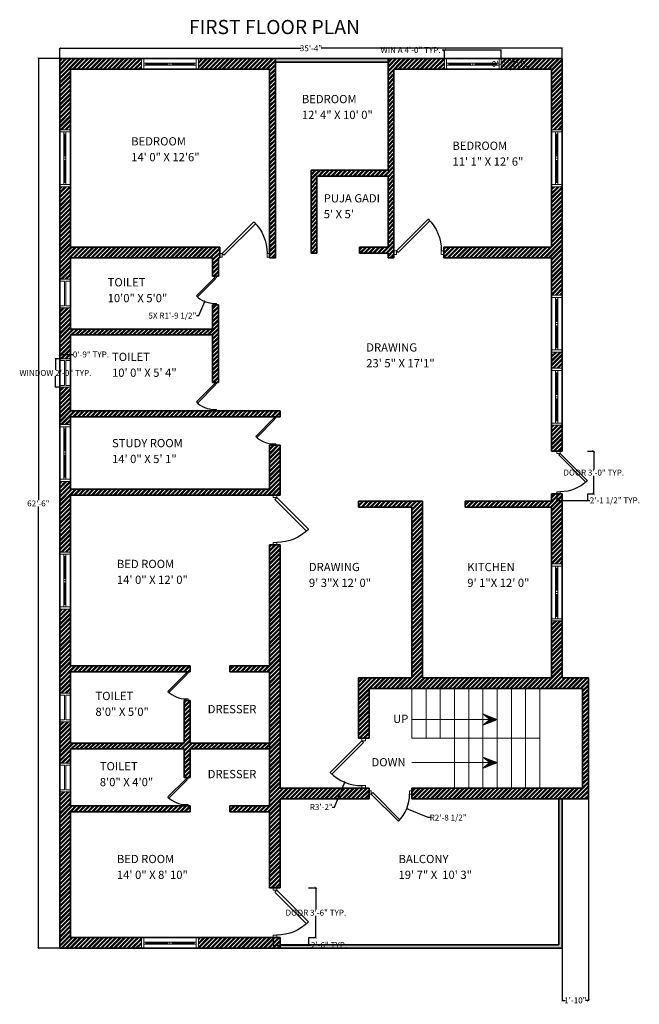
# Model space of a CAD drawing. Units: inches. Extents: x 782 to 2660, y -1008 to 166.
# Tile 12 of 12: x 2137 to 2660, y -752 to 78. Entities that reach past the tile are written whole.
import ezdxf

# ---------------------------------------------------------------- set-up
doc = ezdxf.new("R2010")
doc.units = ezdxf.units.IN
doc.header["$MEASUREMENT"] = 0
for name, color, linetype, lineweight in [('A-ANNO-DIMS', 4, 'Continuous', 18), ('A-ANNO-SYMB', 4, 'Continuous', 18), ('A-ANNO-TEXT', 4, 'Continuous', 18), ('A-AREA-IDEN', 4, 'Continuous', 18), ('A-Door', 150, 'Continuous', 18), ('A-Glaz', 4, 'Continuous', 18), ('A-WALL', 7, 'Continuous', 35), ('A-WALL-PATT', 8, 'Continuous', 13), ('Stairs', 4, 'Continuous', 18)]:
    doc.layers.add(name, color=color, linetype=linetype, lineweight=lineweight)
doc.layers.add('NET 01', color=8, linetype='Continuous')
doc.styles.get("Standard").update_dxf_attribs({"font": 'arial.ttf'})
doc.dimstyles.get("Standard").update_dxf_attribs({"dimtxt": 5, "dimasz": 2, "dimexe": 0.18, "dimexo": 0.0625, "dimgap": 0.09, "dimtad": 0, "dimtih": 1, "dimtoh": 1, "dimdec": 0, "dimzin": 0, "dimdsep": 46, "dimlunit": 3, "dimtxsty": 'Standard', "dimblk": 'ARCHTICK', "dimcen": 0.09, "dimadec": 0, "dimazin": 0, "dimtfac": 1, "dimtdec": 0, "dimtofl": 0, "dimtmove": 0, "dimatfit": 3, "dimfxl": 1, "dimtolj": 1, "dimtzin": 0, "dimarcsym": 0})

# ---------------------------------------------------------------- blocks, each defined once
blk = doc.blocks.new('A$C592222DF')
at = {"layer": 'A-Door'}
for points in [[(-0.035, -0.035), (-0.672, 0.601), (-0.636, 0.636), (0, 0)], [(-0.95, 0), (-0.95, -0.075), (-0.9, -0.075), (-0.9, 0)], [(0, 0), (0, -0.075), (0.05, -0.075), (0.05, 0)]]:
    blk.add_lwpolyline(points, close=True, dxfattribs=at)
at = {"layer": 'NET 01'}
blk.add_arc((0, 0), 0.9, 135, 180, dxfattribs=at)
blk = doc.blocks.new('_ArchTick')
at = {"color": 0, "linetype": 'ByBlock', "const_width": 0.15}
blk.add_lwpolyline([(-0.5, -0.5), (0.5, 0.5)], dxfattribs=at)
blk = doc.blocks.new('*D18')
at = {"layer": 'A-ANNO-DIMS', "color": 0, "lineweight": -2, "transparency": 16777216}
for p, q in [((2171.03, 45.01), (2152.88, 45.01)), ((2153.06, 45.01), (2153.06, -327.35)), ((2153.06, -704.99), (2153.06, -332.64)), ((2171.03, -704.99), (2152.88, -704.99))]:
    blk.add_line(p, q, dxfattribs=at)
at = {"layer": 'Defpoints', "color": 0, "transparency": 16777216}
for p in [(2171.09, 45.01), (2153.06, -704.99), (2171.09, -704.99)]:
    blk.add_point(p, dxfattribs=at)
at = {"layer": 'A-ANNO-DIMS', "color": 0, "lineweight": -2, "transparency": 16777216, "xscale": 2, "yscale": 2, "zscale": 2}
for p, rotation in [((2153.06, 45.01), 90), ((2153.06, -704.99), 270)]:
    blk.add_blockref('_ArchTick', p, dxfattribs=dict(at, rotation=rotation))
at = {"layer": 'A-ANNO-DIMS', "color": 0, "transparency": 16777216, "insert": (2153.06, -329.99), "char_height": 5, "attachment_point": 5}
blk.add_mtext('\\A1;62\'-6"', dxfattribs=at)
blk = doc.blocks.new('*D19')
at = {"layer": 'A-ANNO-DIMS', "color": 0, "lineweight": -2, "transparency": 16777216}
for p, q in [((2171.09, 45.07), (2171.09, 53.91)), ((2171.09, 53.73), (2374.41, 53.73)), ((2595.09, 53.73), (2391.77, 53.73)), ((2595.09, 45.07), (2595.09, 53.91))]:
    blk.add_line(p, q, dxfattribs=at)
at = {"layer": 'Defpoints', "color": 0, "transparency": 16777216}
for p in [(2595.09, 53.73), (2171.09, 45.01), (2595.09, 45.01)]:
    blk.add_point(p, dxfattribs=at)
at = {"layer": 'A-ANNO-DIMS', "color": 0, "lineweight": -2, "transparency": 16777216, "xscale": 2, "yscale": 2, "zscale": 2, "rotation": 180}
blk.add_blockref('_ArchTick', (2171.09, 53.73), dxfattribs=at)
at = {"layer": 'A-ANNO-DIMS', "color": 0, "lineweight": -2, "transparency": 16777216, "xscale": 2, "yscale": 2, "zscale": 2}
blk.add_blockref('_ArchTick', (2595.09, 53.73), dxfattribs=at)
at = {"layer": 'A-ANNO-DIMS', "color": 0, "transparency": 16777216, "insert": (2383.09, 53.73), "char_height": 5, "attachment_point": 5}
blk.add_mtext('\\A1;35\'-4"', dxfattribs=at)
blk = doc.blocks.new('WIN-48-FRAME-A')
for p, q in [((0, 48), (0, 0)), ((0, 48), (9, 48)), ((9, 48), (0, 48)), ((9, 46.15), (0, 46.15)), ((9, 46.15), (0, 46.15)), ((9, 46.15), (0, 46.15)), ((3.35, 1.85), (3.35, 46.15)), ((5.19, 44.31), (3.35, 44.31)), ((3.9, 44.31), (3.9, 25.85)), ((4.27, 44.31), (4.27, 25.85)), ((4.64, 44.31), (4.64, 25.85)), ((5.19, 1.85), (5.19, 46.15)), ((9, 48), (9, 0)), ((3.35, 25.85), (5.19, 25.85)), ((3.35, 24), (5.19, 24)), ((3.35, 22.15), (5.19, 22.15)), ((3.9, 3.69), (3.9, 22.15)), ((4.27, 3.69), (4.27, 22.15)), ((4.64, 3.69), (4.64, 22.15)), ((9, 1.85), (0, 1.85)), ((9, 1.85), (0, 1.85)), ((0, 0), (9, 0)), ((0, 0), (9, 0)), ((5.19, 3.69), (3.35, 3.69))]:
    blk.add_line(p, q)
blk = doc.blocks.new('WIN-24')
for p, q in [((0, 0), (0, 24)), ((0, 24), (9, 24)), ((0, 22.49), (3.9, 22.49)), ((3.9, 1.51), (3.9, 22.49)), ((5.1, 22.49), (9, 22.49)), ((5.1, 1.51), (5.1, 22.49)), ((9, 24), (9, 0)), ((3.9, 1.51), (0, 1.51)), ((9, 0), (0, 0)), ((9, 1.51), (5.1, 1.51))]:
    blk.add_line(p, q)
blk = doc.blocks.new('STAIR-TRAVEL-ARROW')
h = blk.add_hatch()
h.set_pattern_fill('ANSI31', color=256)
h.set_pattern_definition([(45, (-1279.684, 516.831), (-0.088388348, 0.088388348), [])])
h.paths.add_polyline_path([(60, 9.41), (65.9, 4.71), (60, 0), (72, 4.71)])
for p, q in [((65.9, 4.71), (60, 9.41)), ((60, 9.41), (72, 4.71)), ((0, 4.71), (65.9, 4.71)), ((65.9, 4.71), (60, 0)), ((60, 0), (72, 4.71))]:
    blk.add_line(p, q)
blk = doc.blocks.new('*D27')
at = {"layer": 'A-ANNO-DIMS', "color": 0, "lineweight": -2, "transparency": 16777216}
for p, q in [((2380.96, -653.99), (2387.37, -653.99)), ((2387.19, -653.99), (2387.19, -672.31)), ((2387.19, -695.99), (2387.19, -677.67)), ((2380.96, -695.99), (2387.37, -695.99))]:
    blk.add_line(p, q, dxfattribs=at)
at = {"layer": 'Defpoints', "color": 0, "transparency": 16777216}
for p in [(2380.89, -653.99), (2387.19, -653.99), (2380.89, -695.99)]:
    blk.add_point(p, dxfattribs=at)
at = {"layer": 'A-ANNO-DIMS', "color": 0, "lineweight": -2, "transparency": 16777216, "xscale": 2, "yscale": 2, "zscale": 2}
for p, rotation in [((2387.19, -653.99), 90), ((2387.19, -695.99), 270)]:
    blk.add_blockref('_ArchTick', p, dxfattribs=dict(at, rotation=rotation))
at = {"layer": 'A-ANNO-DIMS', "color": 0, "transparency": 16777216, "insert": (2387.19, -674.99), "char_height": 5, "attachment_point": 5}
blk.add_mtext('\\A1;DOOR 3\'-6" TYP.', dxfattribs=at)
blk = doc.blocks.new('*D28')
at = {"layer": 'A-ANNO-DIMS', "color": 0, "lineweight": -2, "transparency": 16777216}
for p, q in [((2351.02, -696.06), (2351.02, -702.47)), ((2380.89, -696.06), (2380.89, -702.47)), ((2351.02, -702.29), (2380.89, -702.29)), ((2380.89, -702.29), (2382.89, -702.29))]:
    blk.add_line(p, q, dxfattribs=at)
at = {"layer": 'Defpoints', "color": 0, "transparency": 16777216}
for p in [(2351.02, -695.99), (2380.89, -695.99), (2380.89, -702.29)]:
    blk.add_point(p, dxfattribs=at)
at = {"layer": 'A-ANNO-DIMS', "color": 0, "lineweight": -2, "transparency": 16777216, "xscale": 2, "yscale": 2, "zscale": 2, "rotation": 180}
blk.add_blockref('_ArchTick', (2351.02, -702.29), dxfattribs=at)
at = {"layer": 'A-ANNO-DIMS', "color": 0, "lineweight": -2, "transparency": 16777216, "xscale": 2, "yscale": 2, "zscale": 2}
blk.add_blockref('_ArchTick', (2380.89, -702.29), dxfattribs=at)
at = {"layer": 'A-ANNO-DIMS', "color": 0, "transparency": 16777216, "insert": (2398.27, -702.29), "char_height": 5, "attachment_point": 5}
blk.add_mtext('\\A1;2\'-6" TYP.', dxfattribs=at)
blk = doc.blocks.new('*D31')
at = {"layer": 'A-ANNO-DIMS', "color": 0, "lineweight": -2, "transparency": 16777216}
for p, q in [((2616.26, -285.99), (2621.78, -285.99)), ((2621.6, -285.99), (2621.6, -301.31)), ((2621.6, -321.99), (2621.6, -306.67)), ((2616.26, -321.99), (2621.78, -321.99))]:
    blk.add_line(p, q, dxfattribs=at)
at = {"layer": 'Defpoints', "color": 0, "transparency": 16777216}
for p in [(2616.2, -285.99), (2621.6, -285.99), (2616.2, -321.99)]:
    blk.add_point(p, dxfattribs=at)
at = {"layer": 'A-ANNO-DIMS', "color": 0, "lineweight": -2, "transparency": 16777216, "xscale": 2, "yscale": 2, "zscale": 2}
for p, rotation in [((2621.6, -285.99), 90), ((2621.6, -321.99), 270)]:
    blk.add_blockref('_ArchTick', p, dxfattribs=dict(at, rotation=rotation))
at = {"layer": 'A-ANNO-DIMS', "color": 0, "transparency": 16777216, "insert": (2621.6, -303.99), "char_height": 5, "attachment_point": 5}
blk.add_mtext('\\A1;DOOR 3\'-0" TYP.', dxfattribs=at)
blk = doc.blocks.new('*D32')
at = {"layer": 'A-ANNO-DIMS', "color": 0, "lineweight": -2, "transparency": 16777216}
for p, q in [((2590.59, -322.06), (2590.59, -327.57)), ((2616.2, -322.06), (2616.2, -327.57)), ((2590.59, -327.39), (2616.2, -327.39)), ((2616.2, -327.39), (2618.2, -327.39))]:
    blk.add_line(p, q, dxfattribs=at)
at = {"layer": 'Defpoints', "color": 0, "transparency": 16777216}
for p in [(2590.59, -321.99), (2616.2, -321.99), (2616.2, -327.39)]:
    blk.add_point(p, dxfattribs=at)
at = {"layer": 'A-ANNO-DIMS', "color": 0, "lineweight": -2, "transparency": 16777216, "xscale": 2, "yscale": 2, "zscale": 2, "rotation": 180}
blk.add_blockref('_ArchTick', (2590.59, -327.39), dxfattribs=at)
at = {"layer": 'A-ANNO-DIMS', "color": 0, "lineweight": -2, "transparency": 16777216, "xscale": 2, "yscale": 2, "zscale": 2}
blk.add_blockref('_ArchTick', (2616.2, -327.39), dxfattribs=at)
at = {"layer": 'A-ANNO-DIMS', "color": 0, "transparency": 16777216, "insert": (2639.4, -327.39), "char_height": 5, "attachment_point": 5}
blk.add_mtext('\\A1;2\'-1 1/2" TYP.', dxfattribs=at)
blk = doc.blocks.new('*D35')
at = {"layer": 'A-ANNO-DIMS', "color": 0, "lineweight": -2, "transparency": 16777216}
for p, q in [((2495.59, 52.21), (2493.59, 52.21)), ((2495.59, 45.07), (2495.59, 52.39)), ((2543.59, 52.21), (2495.59, 52.21)), ((2543.59, 45.07), (2543.59, 52.39))]:
    blk.add_line(p, q, dxfattribs=at)
at = {"layer": 'Defpoints', "color": 0, "transparency": 16777216}
for p in [(2495.59, 52.21), (2495.59, 45.01), (2543.59, 45.01)]:
    blk.add_point(p, dxfattribs=at)
at = {"layer": 'A-ANNO-DIMS', "color": 0, "lineweight": -2, "transparency": 16777216, "xscale": 2, "yscale": 2, "zscale": 2, "rotation": 180.0000000000006}
blk.add_blockref('_ArchTick', (2495.59, 52.21), dxfattribs=at)
at = {"layer": 'A-ANNO-DIMS', "color": 0, "lineweight": -2, "transparency": 16777216, "xscale": 2, "yscale": 2, "zscale": 2}
blk.add_blockref('_ArchTick', (2543.59, 52.21), dxfattribs=at)
at = {"layer": 'A-ANNO-DIMS', "color": 0, "transparency": 16777216, "insert": (2467.1, 52.21), "char_height": 5, "attachment_point": 5}
blk.add_mtext('\\A1;WIN A 4\'-0" TYP.', dxfattribs=at)
blk = doc.blocks.new('*D36')
at = {"layer": 'A-ANNO-DIMS', "color": 0, "lineweight": -2, "transparency": 16777216}
for p, q in [((2543.65, 45.01), (2550.97, 45.01)), ((2550.79, 45.01), (2550.79, 43.15)), ((2543.65, 36.01), (2550.97, 36.01)), ((2550.79, 36.01), (2550.79, 37.86))]:
    blk.add_line(p, q, dxfattribs=at)
at = {"layer": 'Defpoints', "color": 0, "transparency": 16777216}
for p in [(2543.59, 45.01), (2550.79, 45.01), (2543.59, 36.01)]:
    blk.add_point(p, dxfattribs=at)
at = {"layer": 'A-ANNO-DIMS', "color": 0, "lineweight": -2, "transparency": 16777216, "xscale": 2, "yscale": 2, "zscale": 2}
for p, rotation in [((2550.79, 45.01), 90), ((2550.79, 36.01), 270)]:
    blk.add_blockref('_ArchTick', p, dxfattribs=dict(at, rotation=rotation))
at = {"layer": 'A-ANNO-DIMS', "color": 0, "transparency": 16777216, "insert": (2550.79, 40.51), "char_height": 5, "attachment_point": 5}
blk.add_mtext('\\A1;0\'-9" TYP.', dxfattribs=at)
blk = doc.blocks.new('*D39')
at = {"layer": 'A-ANNO-DIMS', "color": 0, "lineweight": -2, "transparency": 16777216}
for p, q in [((2171.03, -207.99), (2167.31, -207.99)), ((2167.49, -207.99), (2167.49, -217.32)), ((2167.49, -231.99), (2167.49, -222.67)), ((2171.03, -231.99), (2167.31, -231.99))]:
    blk.add_line(p, q, dxfattribs=at)
at = {"layer": 'Defpoints', "color": 0, "transparency": 16777216}
for p in [(2167.49, -207.99), (2171.09, -207.99), (2171.09, -231.99)]:
    blk.add_point(p, dxfattribs=at)
at = {"layer": 'A-ANNO-DIMS', "color": 0, "lineweight": -2, "transparency": 16777216, "xscale": 2, "yscale": 2, "zscale": 2}
for p, rotation in [((2167.49, -207.99), 90), ((2167.49, -231.99), 270)]:
    blk.add_blockref('_ArchTick', p, dxfattribs=dict(at, rotation=rotation))
at = {"layer": 'A-ANNO-DIMS', "color": 0, "transparency": 16777216, "insert": (2167.49, -219.99), "char_height": 5, "attachment_point": 5}
blk.add_mtext('\\A1;WINDOW 2\'-0" TYP.', dxfattribs=at)
blk = doc.blocks.new('*D40')
at = {"layer": 'A-ANNO-DIMS', "color": 0, "lineweight": -2, "transparency": 16777216}
for p, q in [((2171.09, -207.93), (2171.09, -204.21)), ((2171.09, -204.39), (2180.09, -204.39)), ((2180.09, -207.93), (2180.09, -204.21)), ((2180.09, -204.39), (2182.09, -204.39))]:
    blk.add_line(p, q, dxfattribs=at)
at = {"layer": 'Defpoints', "color": 0, "transparency": 16777216}
for p in [(2180.09, -204.39), (2171.09, -207.99), (2180.09, -207.99)]:
    blk.add_point(p, dxfattribs=at)
at = {"layer": 'A-ANNO-DIMS', "color": 0, "lineweight": -2, "transparency": 16777216, "xscale": 2, "yscale": 2, "zscale": 2, "rotation": 180}
blk.add_blockref('_ArchTick', (2171.09, -204.39), dxfattribs=at)
at = {"layer": 'A-ANNO-DIMS', "color": 0, "lineweight": -2, "transparency": 16777216, "xscale": 2, "yscale": 2, "zscale": 2}
blk.add_blockref('_ArchTick', (2180.09, -204.39), dxfattribs=at)
at = {"layer": 'A-ANNO-DIMS', "color": 0, "transparency": 16777216, "insert": (2197.42, -204.39), "char_height": 5, "attachment_point": 5}
blk.add_mtext('\\A1;0\'-9" TYP.', dxfattribs=at)
blk = doc.blocks.new('*D54')
at = {"layer": 'A-ANNO-DIMS', "color": 0, "lineweight": -2, "transparency": 16777216}
for p, q in [((2595.09, -579.06), (2595.09, -749.12)), ((2617.09, -579.06), (2617.09, -749.12)), ((2595.09, -748.94), (2597.65, -748.94)), ((2617.09, -748.94), (2614.53, -748.94))]:
    blk.add_line(p, q, dxfattribs=at)
at = {"layer": 'Defpoints', "color": 0, "transparency": 16777216}
for p in [(2595.09, -578.99), (2617.09, -578.99), (2617.09, -748.94)]:
    blk.add_point(p, dxfattribs=at)
at = {"layer": 'A-ANNO-DIMS', "color": 0, "lineweight": -2, "transparency": 16777216, "xscale": 2, "yscale": 2, "zscale": 2, "rotation": 180}
blk.add_blockref('_ArchTick', (2595.09, -748.94), dxfattribs=at)
at = {"layer": 'A-ANNO-DIMS', "color": 0, "lineweight": -2, "transparency": 16777216, "xscale": 2, "yscale": 2, "zscale": 2}
blk.add_blockref('_ArchTick', (2617.09, -748.94), dxfattribs=at)
at = {"layer": 'A-ANNO-DIMS', "color": 0, "transparency": 16777216, "insert": (2606.09, -748.94), "char_height": 5, "attachment_point": 5}
blk.add_mtext('\\A1;1\'-10"', dxfattribs=at)
blk = doc.blocks.new('*D64')
at = {"layer": 'A-ANNO-DIMS', "color": 0, "lineweight": -2, "transparency": 16777216}
for p, q in [((2425.93, -530.09), (2426.11, -530.09)), ((2426.02, -530.18), (2426.02, -530)), ((2402.87, -585.97), (2411.55, -565.02)), ((2400.87, -585.97), (2402.87, -585.97))]:
    blk.add_line(p, q, dxfattribs=at)
at = {"layer": 'Defpoints', "color": 0, "transparency": 16777216}
for p in [(2426.02, -530.09), (2411.55, -565.02)]:
    blk.add_point(p, dxfattribs=at)
at = {"layer": 'A-ANNO-DIMS', "color": 0, "lineweight": -2, "transparency": 16777216, "xscale": 2, "yscale": 2, "zscale": 2, "rotation": 67.50012386057699}
blk.add_blockref('_ArchTick', (2411.55, -565.02), dxfattribs=at)
at = {"layer": 'A-ANNO-DIMS', "color": 0, "transparency": 16777216, "insert": (2391.74, -585.97), "char_height": 5, "attachment_point": 5}
blk.add_mtext('\\A1;R3\'-2"', dxfattribs=at)
blk = doc.blocks.new('*D65')
at = {"layer": 'A-ANNO-DIMS', "color": 0, "lineweight": -2, "transparency": 16777216}
for p, q in [((2433.8, -574.98), (2433.98, -574.98)), ((2433.89, -575.07), (2433.89, -574.89)), ((2481.78, -594.82), (2463.82, -587.38)), ((2483.78, -594.82), (2481.78, -594.82))]:
    blk.add_line(p, q, dxfattribs=at)
at = {"layer": 'Defpoints', "color": 0, "transparency": 16777216}
for p in [(2433.89, -574.98), (2463.82, -587.38)]:
    blk.add_point(p, dxfattribs=at)
at = {"layer": 'A-ANNO-DIMS', "color": 0, "lineweight": -2, "transparency": 16777216, "xscale": 2, "yscale": 2, "zscale": 2, "rotation": 157.4994644813111}
blk.add_blockref('_ArchTick', (2463.82, -587.38), dxfattribs=at)
at = {"layer": 'A-ANNO-DIMS', "color": 0, "transparency": 16777216, "insert": (2498.74, -594.82), "char_height": 5, "attachment_point": 5}
blk.add_mtext('\\A1;R2\'-8 1/2"', dxfattribs=at)
blk = doc.blocks.new('*D66')
at = {"layer": 'A-ANNO-DIMS', "color": 0, "lineweight": -2, "transparency": 16777216}
for p, q in [((2301.6, -139.73), (2301.78, -139.73)), ((2301.69, -139.82), (2301.69, -139.64)), ((2288.47, -171.66), (2293.43, -159.69)), ((2286.47, -171.66), (2288.47, -171.66))]:
    blk.add_line(p, q, dxfattribs=at)
at = {"layer": 'Defpoints', "color": 0, "transparency": 16777216}
for p in [(2301.69, -139.73), (2293.43, -159.69)]:
    blk.add_point(p, dxfattribs=at)
at = {"layer": 'A-ANNO-DIMS', "color": 0, "lineweight": -2, "transparency": 16777216, "xscale": 2, "yscale": 2, "zscale": 2, "rotation": 67.49981965550745}
blk.add_blockref('_ArchTick', (2293.43, -159.69), dxfattribs=at)
at = {"layer": 'A-ANNO-DIMS', "color": 0, "transparency": 16777216, "insert": (2266.14, -171.66), "char_height": 5, "attachment_point": 5}
blk.add_mtext('\\A1;5X R1\'-9 1/2"', dxfattribs=at)

msp = doc.modelspace()

# ---------------------------------------------------------------- hatches: boundary and pattern name
at = {"layer": 'A-WALL-PATT'}
h = msp.add_hatch(dxfattribs=at)
h.set_pattern_fill('ANSI32', color=256, scale=7)
h.paths.add_polyline_path([(2240.09, 45.01), (2171.09, 45.01), (2171.09, -14.99), (2180.09, -14.99), (2180.09, 36.01), (2240.09, 36.01)])
h.paths.add_polyline_path([(2180.09, -62.99), (2171.09, -62.99), (2171.09, -140.99), (2180.09, -140.99), (2180.09, -122.99), (2300.09, -122.99), (2300.09, -138.53), (2305.09, -138.53), (2305.09, -122.99), (2306.09, -122.99), (2306.09, -113.99), (2180.09, -113.99)])
h.paths.add_polyline_path([(2305.09, -162.53), (2300.09, -162.53), (2300.09, -182.99), (2180.09, -182.99), (2180.09, -164.99), (2171.09, -164.99), (2171.09, -207.99), (2180.09, -207.99), (2180.09, -187.99), (2300.09, -187.99), (2300.09, -227.99), (2305.09, -227.99)])
h.paths.add_polyline_path([(2180.09, -231.99), (2171.09, -231.99), (2171.09, -263.49), (2180.09, -263.49), (2180.09, -256.99), (2305.09, -256.99), (2348.09, -256.99), (2357.09, -256.99), (2357.09, -251.99), (2305.09, -251.99), (2300.09, -251.99), (2180.09, -251.99)])
h.paths.add_polyline_path([(2180.09, -322.99), (2348.09, -322.99), (2357.09, -322.99), (2357.09, -280.99), (2348.09, -280.99), (2348.09, -317.99), (2180.09, -317.99), (2180.09, -311.49), (2171.09, -311.49), (2171.09, -370.99), (2180.09, -370.99)])
h.paths.add_polyline_path([(2180.09, -418.99), (2171.09, -418.99), (2171.09, -489.99), (2180.09, -489.99), (2180.09, -471.99), (2276.09, -471.99), (2281.09, -471.99), (2281.09, -466.99), (2180.09, -466.99)])
h.paths.add_polyline_path([(2180.09, -513.99), (2171.09, -513.99), (2171.09, -548.99), (2180.09, -548.99), (2180.09, -536.99), (2276.09, -536.99), (2276.09, -560.99), (2281.09, -560.99), (2281.09, -536.99), (2348.09, -536.99), (2348.09, -531.99), (2281.09, -531.99), (2281.09, -495.99), (2276.09, -495.99), (2276.09, -531.99), (2180.09, -531.99)])
h.paths.add_polyline_path([(2281.09, -584.99), (2276.09, -584.99), (2180.09, -584.99), (2180.09, -572.99), (2171.09, -572.99), (2171.09, -704.99), (2240.09, -704.99), (2240.09, -695.99), (2180.09, -695.99), (2180.09, -589.99), (2281.09, -589.99)])
h.paths.add_polyline_path([(2357.09, -695.99), (2348.09, -695.99), (2288.09, -695.99), (2288.09, -704.99), (2357.09, -704.99)])
h.paths.add_polyline_path([(2357.09, -578.99), (2432.09, -578.99), (2432.09, -569.99), (2357.09, -569.99), (2357.09, -364.99), (2348.09, -364.99), (2348.09, -466.99), (2314.59, -466.99), (2314.59, -471.99), (2348.09, -471.99), (2348.09, -584.99), (2314.59, -584.99), (2314.59, -589.99), (2348.09, -589.99), (2348.09, -653.99), (2357.09, -653.99)])
h.paths.add_polyline_path([(2477.09, -332.99), (2477.09, -327.99), (2453.09, -327.99), (2423.09, -327.99), (2423.09, -332.99), (2453.09, -332.99), (2468.09, -332.99), (2468.09, -476.99), (2423.09, -476.99), (2423.09, -485.99), (2423.09, -527.99), (2432.09, -527.99), (2432.09, -485.99), (2595.09, -485.99), (2612.09, -485.99), (2612.09, -569.99), (2468.09, -569.99), (2468.09, -578.99), (2592.09, -578.99), (2595.09, -578.99), (2617.09, -578.99), (2617.09, -476.99), (2595.09, -476.99), (2595.09, -428.99), (2586.09, -428.99), (2586.09, -476.99), (2477.09, -476.99)])
h.paths.add_polyline_path([(2595.09, -321.99), (2586.09, -321.99), (2586.09, -327.99), (2513.09, -327.99), (2513.09, -332.99), (2586.09, -332.99), (2586.09, -380.99), (2595.09, -380.99)])
h.paths.add_polyline_path([(2595.09, -264.07), (2586.09, -264.07), (2586.09, -285.99), (2595.09, -285.99)])
h.paths.add_polyline_path([(2595.09, -202.4), (2586.09, -202.4), (2586.09, -216.07), (2595.09, -216.07)])
h.paths.add_polyline_path([(2595.09, -62.99), (2586.09, -62.99), (2586.09, -113.99), (2495.09, -113.99), (2495.09, -122.99), (2586.09, -122.99), (2586.09, -154.4), (2595.09, -154.4)])
h.paths.add_polyline_path([(2595.09, 45.01), (2543.59, 45.01), (2543.59, 36.01), (2586.09, 36.01), (2586.09, -14.99), (2595.09, -14.99)])
h.paths.add_polyline_path([(2495.59, 45.01), (2448.09, 45.01), (2448.09, -48.99), (2383.09, -48.99), (2383.09, -118.99), (2388.09, -118.99), (2388.09, -53.99), (2448.09, -53.99), (2448.09, -113.99), (2424.09, -113.99), (2424.09, -118.99), (2448.09, -118.99), (2448.09, -122.99), (2453.09, -122.99), (2453.09, -113.99), (2453.09, 36.01), (2495.59, 36.01)])
h.paths.add_polyline_path([(2353.09, 45.01), (2288.09, 45.01), (2288.09, 36.01), (2348.09, 36.01), (2348.09, -113.99), (2348.09, -122.99), (2353.09, -122.99), (2353.09, -118.99)])
h = msp.add_hatch(color=256, dxfattribs=at)
h.dxf.hatch_style = 1
h.paths.add_polyline_path([(2448.09, 45.01), (2353.09, 45.01), (2353.09, 42.01), (2448.09, 42.01)])
h.paths.add_polyline_path([(2595.09, -578.99), (2592.09, -578.99), (2592.09, -701.99), (2357.09, -701.99), (2357.09, -704.99), (2586.09, -704.99), (2595.09, -704.99)])

# ---------------------------------------------------------------- linework, layer by layer
at = {"layer": 'A-WALL'}
for p, q in [((2171.09, 45.01), (2171.09, -704.99)), ((2171.09, 45.01), (2595.09, 45.01)), ((2353.09, 45.01), (2353.09, -122.99)), ((2353.09, 42.01), (2448.09, 42.01)), ((2448.09, 45.01), (2448.09, -48.99)), ((2595.09, 45.01), (2595.09, -285.99)), ((2180.09, 36.01), (2348.09, 36.01)), ((2180.09, 36.01), (2180.09, -113.99)), ((2348.09, 36.01), (2348.09, -113.99)), ((2453.09, 36.01), (2586.09, 36.01)), ((2453.09, 36.01), (2453.09, -113.99)), ((2453.09, 36.01), (2586.09, 36.01)), ((2586.09, 36.01), (2586.09, -113.99)), ((2383.09, -48.99), (2448.09, -48.99)), ((2383.09, -48.99), (2383.09, -118.99)), ((2388.09, -53.99), (2448.09, -53.99)), ((2388.09, -53.99), (2388.09, -118.99)), ((2448.09, -53.99), (2448.09, -113.99)), ((2180.09, -113.99), (2306.09, -113.99)), ((2306.09, -113.99), (2306.09, -122.99)), ((2348.09, -113.99), (2348.09, -122.99)), ((2424.09, -118.99), (2424.09, -113.99)), ((2424.09, -113.99), (2448.09, -113.99)), ((2453.09, -113.99), (2453.09, -122.99)), ((2495.09, -113.99), (2586.09, -113.99)), ((2495.09, -113.99), (2495.09, -122.99)), ((2180.09, -122.99), (2300.09, -122.99)), ((2180.09, -122.99), (2180.09, -182.99)), ((2300.09, -122.99), (2300.09, -138.53)), ((2305.09, -122.99), (2305.09, -138.53)), ((2305.09, -122.99), (2306.09, -122.99)), ((2348.09, -122.99), (2353.09, -122.99)), ((2353.09, -118.99), (2353.09, -122.99)), ((2383.09, -118.99), (2388.09, -118.99)), ((2424.09, -118.99), (2448.09, -118.99)), ((2448.09, -118.99), (2448.09, -122.99)), ((2448.09, -122.99), (2453.09, -122.99)), ((2495.09, -122.99), (2586.09, -122.99)), ((2586.09, -122.99), (2586.09, -285.99)), ((2300.09, -138.53), (2305.09, -138.53)), ((2300.09, -162.53), (2305.09, -162.53)), ((2300.09, -162.53), (2300.09, -182.99)), ((2305.09, -162.53), (2305.09, -227.99)), ((2180.09, -182.99), (2300.09, -182.99)), ((2180.09, -187.99), (2300.09, -187.99)), ((2180.09, -187.99), (2180.09, -251.99)), ((2300.09, -187.99), (2300.09, -227.99)), ((2300.09, -227.99), (2305.09, -227.99)), ((2180.09, -251.99), (2300.09, -251.99)), ((2180.09, -256.99), (2305.09, -256.99)), ((2180.09, -256.99), (2180.09, -317.99)), ((2300.09, -251.99), (2305.09, -251.99)), ((2305.09, -251.99), (2357.09, -251.99)), ((2305.09, -256.99), (2348.09, -256.99)), ((2348.09, -256.99), (2357.09, -256.99)), ((2357.09, -256.99), (2357.09, -251.99)), ((2348.09, -280.99), (2348.09, -317.99)), ((2348.09, -280.99), (2357.09, -280.99)), ((2357.09, -280.99), (2357.09, -322.99)), ((2586.09, -285.99), (2595.09, -285.99)), ((2180.09, -317.99), (2348.09, -317.99)), ((2180.09, -322.99), (2348.09, -322.99)), ((2180.09, -322.99), (2180.09, -466.99)), ((2348.09, -322.99), (2357.09, -322.99)), ((2586.09, -321.99), (2595.09, -321.99)), ((2586.09, -321.99), (2586.09, -327.99)), ((2586.09, -321.99), (2586.09, -327.99)), ((2595.09, -321.99), (2595.09, -476.99)), ((2423.09, -327.99), (2453.09, -327.99)), ((2423.09, -332.99), (2423.09, -327.99)), ((2453.09, -327.99), (2477.09, -327.99)), ((2477.09, -332.99), (2477.09, -327.99)), ((2513.09, -327.99), (2586.09, -327.99)), ((2513.09, -332.99), (2513.09, -327.99)), ((2423.09, -332.99), (2453.09, -332.99)), ((2453.09, -332.99), (2468.09, -332.99)), ((2468.09, -332.99), (2468.09, -476.99)), ((2477.09, -332.99), (2477.09, -476.99)), ((2513.09, -332.99), (2586.09, -332.99)), ((2586.09, -332.99), (2586.09, -476.99)), ((2348.09, -364.99), (2357.09, -364.99)), ((2348.09, -364.99), (2348.09, -466.99)), ((2357.09, -364.99), (2357.09, -569.99)), ((2180.09, -466.99), (2281.09, -466.99)), ((2180.09, -471.99), (2276.09, -471.99)), ((2180.09, -471.99), (2180.09, -531.99)), ((2276.09, -471.99), (2281.09, -471.99)), ((2281.09, -471.99), (2281.09, -466.99)), ((2314.59, -471.99), (2314.59, -466.99)), ((2314.59, -466.99), (2348.09, -466.99)), ((2314.59, -471.99), (2348.09, -471.99)), ((2348.09, -471.99), (2348.09, -584.99)), ((2423.09, -476.99), (2468.09, -476.99)), ((2423.09, -476.99), (2423.09, -485.99)), ((2477.09, -476.99), (2586.09, -476.99)), ((2595.09, -476.99), (2617.09, -476.99)), ((2617.09, -476.99), (2617.09, -578.99)), ((2423.09, -485.99), (2423.09, -527.99)), ((2432.09, -485.99), (2595.09, -485.99)), ((2432.09, -485.99), (2432.09, -527.99)), ((2453.09, -485.99), (2612.09, -485.99)), ((2612.09, -485.99), (2612.09, -569.99)), ((2276.09, -495.99), (2276.09, -531.99)), ((2276.09, -495.99), (2281.09, -495.99)), ((2281.09, -495.99), (2281.09, -531.99)), ((2432.09, -527.99), (2423.09, -527.99)), ((2180.09, -531.99), (2276.09, -531.99)), ((2180.09, -536.99), (2276.09, -536.99)), ((2180.09, -536.99), (2180.09, -584.99)), ((2276.09, -536.99), (2276.09, -560.99)), ((2281.09, -531.99), (2348.09, -531.99)), ((2281.09, -536.99), (2281.09, -560.99)), ((2281.09, -536.99), (2348.09, -536.99)), ((2276.09, -560.99), (2281.09, -560.99)), ((2357.09, -569.99), (2432.09, -569.99)), ((2432.09, -569.99), (2432.09, -578.99)), ((2468.09, -569.99), (2468.09, -578.99)), ((2468.09, -569.99), (2612.09, -569.99)), ((2357.09, -578.99), (2432.09, -578.99)), ((2357.09, -578.99), (2357.09, -653.99)), ((2468.09, -578.99), (2592.09, -578.99)), ((2592.09, -701.99), (2592.09, -578.99)), ((2592.09, -578.99), (2595.09, -578.99)), ((2595.09, -578.99), (2617.09, -578.99)), ((2595.09, -704.99), (2595.09, -578.99)), ((2180.09, -584.99), (2276.09, -584.99)), ((2276.09, -584.99), (2281.09, -584.99)), ((2281.09, -584.99), (2281.09, -589.99)), ((2314.59, -584.99), (2348.09, -584.99)), ((2314.59, -584.99), (2314.59, -589.99)), ((2180.09, -589.99), (2281.09, -589.99)), ((2180.09, -589.99), (2180.09, -695.99)), ((2314.59, -589.99), (2348.09, -589.99)), ((2348.09, -589.99), (2348.09, -653.99)), ((2348.09, -653.99), (2357.09, -653.99)), ((2348.09, -695.99), (2180.09, -695.99)), ((2348.09, -695.99), (2357.09, -695.99)), ((2357.09, -695.99), (2357.09, -704.99)), ((2586.09, -704.99), (2171.09, -704.99)), ((2592.09, -701.99), (2357.09, -701.99)), ((2586.09, -704.99), (2595.09, -704.99))]:
    msp.add_line(p, q, dxfattribs=at)
at = {"layer": 'Stairs'}
for p, q in [((2468.09, -485.99), (2468.09, -527.99)), ((2480.09, -485.99), (2480.09, -527.99)), ((2492.09, -485.99), (2492.09, -527.99)), ((2504.09, -485.99), (2504.09, -569.99)), ((2516.09, -485.99), (2516.09, -569.99)), ((2528.09, -485.99), (2528.09, -569.99)), ((2540.09, -485.99), (2540.09, -569.99)), ((2552.09, -485.99), (2552.09, -569.99)), ((2564.09, -485.99), (2564.09, -569.99)), ((2576.09, -485.99), (2576.09, -569.99)), ((2576.09, -527.99), (2468.09, -527.99))]:
    msp.add_line(p, q, dxfattribs=at)

# ---------------------------------------------------------------- block references
at = {"layer": 'A-ANNO-SYMB'}
for p in [(2468.09, -516.83), (2468.09, -553.17)]:
    msp.add_blockref('STAIR-TRAVEL-ARROW', p, dxfattribs=at)
at = {"layer": 'A-Door', "xscale": -42, "yscale": 42, "zscale": 42}
for p in [(2455.19, -116.92), (2308.19, -119.24)]:
    msp.add_blockref('A$C592222DF', p, dxfattribs=at)
at = {"layer": 'A-Door'}
for p, xscale, yscale, zscale, rotation in [((2301.69, -139.73), 24, 24, 24, 90), ((2301.69, -229.19), 24, 24, 24, 90), ((2351.69, -258.19), 24, 24, 24, 90), ((2593.29, -287.79), -36, 36, 36, 270), ((2354.17, -325.09), -42, 42, 42, 270), ((2277.69, -473.19), 24, 24, 24, 90), ((2426.02, -530.09), 42, 42, 42, 90.00000000000003), ((2277.69, -562.19), 24, 24, 24, 90), ((2433.89, -574.98), 36.00000000000091, 36.00000000000091, 36.00000000000091, 180), ((2354.17, -656.09), -42, 42, 42, 270)]:
    msp.add_blockref('A$C592222DF', p, dxfattribs=dict(at, xscale=xscale, yscale=yscale, zscale=zscale, rotation=rotation))
at = {"layer": 'A-Glaz'}
for p, rotation in [((2288.09, 36.01), 90.00000000000055), ((2543.59, 36.01), 90.00000000000055), ((2288.09, -704.99), 89.99999999999896)]:
    msp.add_blockref('WIN-48-FRAME-A', p, dxfattribs=dict(at, rotation=rotation))
for name, p in [('WIN-48-FRAME-A', (2171.09, -62.99)), ('WIN-48-FRAME-A', (2586.09, -62.99)), ('WIN-24', (2171.09, -164.99)), ('WIN-48-FRAME-A', (2586.09, -202.4)), ('WIN-24', (2171.09, -231.99)), ('WIN-48-FRAME-A', (2586.09, -264.07)), ('WIN-48-FRAME-A', (2171.09, -311.49)), ('WIN-48-FRAME-A', (2171.09, -418.99)), ('WIN-48-FRAME-A', (2586.09, -428.99)), ('WIN-24', (2171.09, -513.99)), ('WIN-24', (2171.09, -572.99))]:
    msp.add_blockref(name, p, dxfattribs=at)

# ---------------------------------------------------------------- texts
at = {"layer": 'A-ANNO-TEXT'}
for s, height, p in [('FIRST FLOOR PLAN', 11.9654, (2280.06, 65.64)), ('UP', 6.958, (2452.36, -515.08)), ('DOWN', 6.958, (2434.11, -551.62))]:
    msp.add_text(s, height=height, dxfattribs=at).set_placement(p)
at = {"layer": 'A-AREA-IDEN'}
for s, height, p in [('BEDROOM', 6.958, (2375.37, 7.41)), ('12\' 4" X 10\' 0"', 6.9576, (2375.37, -5.93)), ('BEDROOM', 6.958, (2231.39, -28.18)), ('BEDROOM', 6.958, (2502.4, -31.92)), ('14\' 0" X 12\'6"', 6.9576, (2231.39, -41.52)), ('11\' 1" X 12\' 6"', 6.9576, (2502.4, -45.26)), ('PUJA GADI', 6.958, (2393.81, -76.23)), ("5' X 5' ", 6.958, (2393.81, -89.57)), ('TOILET', 6.958, (2211.52, -147.02)), ('10\'0" X 5\'0" ', 6.9576, (2211.52, -160.36)), ('DRAWING', 6.958, (2429.69, -201.94)), ('TOILET', 6.958, (2215.21, -209.91)), ('23\' 5" X 17\'1"', 6.9576, (2429.69, -215.28)), ('10\' 0" X 5\' 4" ', 6.9576, (2215.21, -223.25)), ('STUDY ROOM', 6.958, (2215.21, -282.63)), ('14\' 0" X 5\' 1" ', 6.9576, (2215.21, -295.97)), ('BED ROOM', 6.958, (2219.35, -384.48)), ('DRAWING', 6.958, (2381.31, -387.05)), ('KITCHEN', 6.958, (2514.9, -387.05)), ('14\' 0" X 12\' 0" ', 6.9576, (2219.35, -397.81)), ('9\' 3"X 12\' 0"', 6.9576, (2381.31, -400.39)), ('9\' 1"X 12\' 0"', 6.9576, (2514.9, -400.39)), ('TOILET', 6.958, (2201.25, -495.75)), ('8\'0" X 5\'0" ', 6.9576, (2201.25, -509.09)), ('DRESSER', 6.958, (2295.92, -506.83)), ('TOILET', 6.958, (2204.93, -555.01)), ('DRESSER', 6.958, (2295.92, -561.61)), ('8\'0" X 4\'0" ', 6.9576, (2204.93, -568.35)), ('BED ROOM', 6.958, (2219.35, -633.2)), ('BALCONY', 6.958, (2456.92, -633.2)), ('14\' 0" X 8\' 10" ', 6.9576, (2219.35, -646.54)), ('19\' 7" X  10\' 3" ', 6.9576, (2456.92, -646.54))]:
    msp.add_text(s, height=height, dxfattribs=at).set_placement(p)

# ---------------------------------------------------------------- dimensions: what is measured, and where the dimension line sits
at = {"layer": 'A-ANNO-DIMS'}
for base, p1, p2, angle, text, picture, middle in [((2495.59, 52.21), (2543.59, 45.01), (2495.59, 45.01), 180, 'WIN A <> TYP.', '*D35', (2467.1, 52.21)), ((2550.79, 45.01), (2543.59, 36.01), (2543.59, 45.01), 90, '<> TYP.', '*D36', (2550.79, 40.51)), ((2167.49, -207.99), (2171.09, -231.99), (2171.09, -207.99), 90, 'WINDOW <> TYP.', '*D39', (2167.49, -219.99)), ((2621.6, -285.99), (2616.2, -321.99), (2616.2, -285.99), 90, 'DOOR <> TYP.', '*D31', (2621.6, -303.99)), ((2387.19, -653.99), (2380.89, -695.99), (2380.89, -653.99), 90, 'DOOR <> TYP.', '*D27', (2387.19, -674.99))]:
    dim = msp.add_linear_dim(base=base, p1=p1, p2=p2, angle=angle, text=text, dimstyle='Standard', override={"dimdec": 1, "dimlfac": 1, "dimrnd": 0, "dimzin": 1, "dimdsep": 46, "dimlunit": 4, "dimfrac": 2}, dxfattribs=at)
    dim.commit()
    dim.dimension.update_dxf_attribs({"geometry": picture, "text_midpoint": middle})
for base, p1, p2, override, picture, middle in [((2595.09, 53.73), (2171.09, 45.01), (2595.09, 45.01), {"dimclrd": 0, "dimclre": 0, "dimclrt": 0}, '*D19', (2383.09, 53.73)), ((2617.09, -748.94), (2595.09, -578.99), (2617.09, -578.99), {"dimdec": 1, "dimlfac": 1, "dimrnd": 0, "dimzin": 1, "dimdsep": 46, "dimlunit": 4, "dimfrac": 2}, '*D54', (2606.09, -748.94))]:
    dim = msp.add_linear_dim(base=base, p1=p1, p2=p2, dimstyle='Standard', override=override, dxfattribs=at)
    dim.commit()
    dim.dimension.update_dxf_attribs({"geometry": picture, "text_midpoint": middle})
dim = msp.add_linear_dim(base=(2153.06, -704.99), p1=(2171.09, 45.01), p2=(2171.09, -704.99), angle=90, dimstyle='Standard', override={"dimclrd": 0, "dimclre": 0, "dimclrt": 0}, dxfattribs=at)
dim.commit()
dim.dimension.update_dxf_attribs({"geometry": '*D18', "text_midpoint": (2153.06, -329.99)})
dim = msp.add_radius_dim(center=(2301.69, -139.73), mpoint=(2293.43, -159.69), text='5X <>', dimstyle='Standard', override={"dimdec": 1, "dimlfac": 1, "dimrnd": 0, "dimzin": 1, "dimdsep": 46, "dimlunit": 4, "dimfrac": 2}, dxfattribs=at)
dim.commit()
dim.dimension.update_dxf_attribs({"geometry": '*D66', "text_midpoint": (2266.14, -171.66), "dimtype": 164})
for base, p1, p2, picture, middle in [((2180.09, -204.39), (2171.09, -207.99), (2180.09, -207.99), '*D40', (2197.42, -204.39)), ((2616.2, -327.39), (2590.59, -321.99), (2616.2, -321.99), '*D32', (2639.4, -327.39)), ((2380.89, -702.29), (2351.02, -695.99), (2380.89, -695.99), '*D28', (2398.27, -702.29))]:
    dim = msp.add_linear_dim(base=base, p1=p1, p2=p2, text='<> TYP.', dimstyle='Standard', override={"dimdec": 1, "dimlfac": 1, "dimrnd": 0, "dimzin": 1, "dimdsep": 46, "dimlunit": 4, "dimfrac": 2}, dxfattribs=at)
    dim.commit()
    dim.dimension.update_dxf_attribs({"geometry": picture, "text_midpoint": middle})
for center, mpoint, picture, middle in [((2426.02, -530.09), (2411.55, -565.02), '*D64', (2391.74, -585.97)), ((2433.89, -574.98), (2463.82, -587.38), '*D65', (2498.74, -594.82))]:
    dim = msp.add_radius_dim(center=center, mpoint=mpoint, dimstyle='Standard', override={"dimdec": 1, "dimlfac": 1, "dimrnd": 0, "dimzin": 1, "dimdsep": 46, "dimlunit": 4, "dimfrac": 2}, dxfattribs=at)
    dim.commit()
    dim.dimension.update_dxf_attribs({"geometry": picture, "text_midpoint": middle, "dimtype": 164})

doc.saveas('drawing.dxf')
